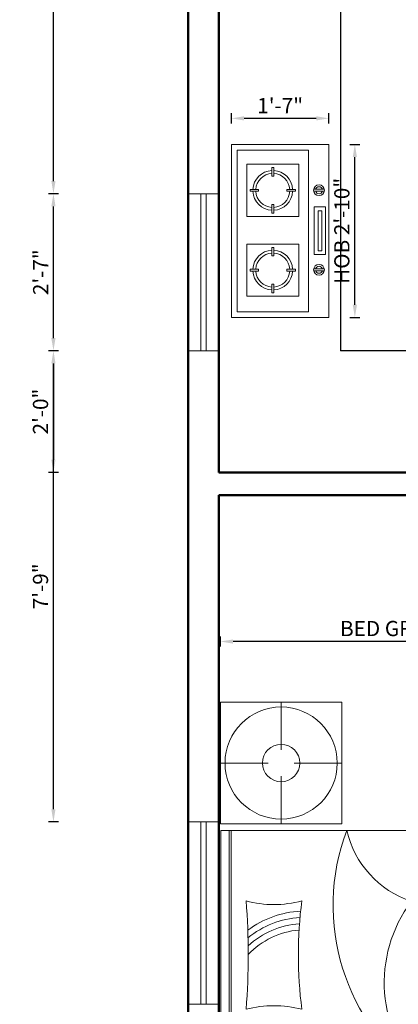
# Model space of a CAD drawing. Units: inches. Extents: x 1961 to 3038, y 800 to 1438.
# Tile 2 of 13: x 2592 to 2666, y 953 to 1148. Entities that reach past the tile are written whole.
import ezdxf

# ---------------------------------------------------------------- set-up
doc = ezdxf.new("R2010")
doc.units = ezdxf.units.IN
for name, color, linetype, lineweight in [('A-ANNO-DIMS', 2, 'Continuous', 18), ('A-EQPM', 8, 'Continuous', 18), ('A-FLOR-CASE', 8, 'Continuous', 25), ('A-FURN', 8, 'Continuous', 18), ('A-GLAZ', 4, 'Continuous', 18), ('A-WALL', 7, 'Continuous', 50)]:
    doc.layers.add(name, color=color, linetype=linetype, lineweight=lineweight)
doc.styles.get("Standard").update_dxf_attribs({"font": 'arial.ttf'})
doc.dimstyles.new('ISO-25', dxfattribs={"dimtxt": 3, "dimasz": 2.5, "dimexe": 1, "dimexo": 1, "dimtad": 1, "dimdec": 4, "dimlunit": 4, "dimtxsty": 'Standard', "dimcen": 2.5, "dimadec": 0, "dimazin": 0, "dimtfac": 1, "dimtdec": 4, "dimtmove": 0, "dimatfit": 3, "dimfxl": 1, "dimfxlon": 1, "dimarcsym": 0})

# ---------------------------------------------------------------- blocks, each defined once
blk = doc.blocks.new('A$C11850ECD')
for p, q in [((0, 1.95), (0, 0.04)), ((0, 1.95), (1.2, 1.95)), ((1.2, 1.95), (1.2, 0.04)), ((1.2318, 1.952), (1.8168, 1.952)), ((1.2318, 1.367), (1.2318, 1.952)), ((1.5243, 1.952), (1.5243, 1.7225)), ((1.8168, 1.952), (1.8168, 1.367)), ((0, 1.91), (1.2, 1.91)), ((0, 1.9), (1.2, 1.9)), ((1.4613, 1.6586), (1.2318, 1.6586)), ((1.8168, 1.6595), (1.5873, 1.6595)), ((1.5243, 1.5965), (1.5243, 1.367)), ((1.8168, 1.367), (1.2318, 1.367)), ((0, 0.58), (1.2, 0.58)), ((0, 0.55), (1.2, 0.55)), ((0, 0.52), (1.2, 0.52)), ((0, 0.49), (1.2, 0.49)), ((0, 0.46), (1.2, 0.46)), ((0, 0.43), (1.2, 0.43)), ((0, 0.4), (1.2, 0.4)), ((1.16, 0), (0.04, 0))]:
    blk.add_line(p, q)
for radius in [0.27, 0.09]:
    blk.add_circle((1.5243, 1.6595), radius)
for centre, radius, start, end in [((-0.2053, 1.694), 0.5605, 346.15, 13.85), ((0.5998, 5.1077), 3.2899, 265.4501, 274.5499), ((0.3425, 1.5416), 0.3789, 4.7708, 46.8165), ((0.3425, 1.5416), 0.4089, 4.1373, 42.5614), ((0.3425, 1.5416), 0.4389, 3.5318, 39.1874), ((0.3425, 1.5416), 0.4689, 2.9489, 36.4321), ((1.3429, 1.694), 0.5004, 164.4468, 195.5532), ((0.5998, -0.4629), 2.0395, 82.6483, 97.3517), ((0.8389, 0.3894), 1.0202, 69.2731, 145.3133), ((1.3044, 0.8859), 0.4695, 102.8515, 161.769), ((0.4655, 0.5058), 0.6574, 53.2823, 135.0802), ((0.04, 0.04), 0.04, 180, 270), ((1.16, 0.04), 0.04, 270, 0)]:
    blk.add_arc(centre, radius, start, end)
blk = doc.blocks.new('A$C056B3B93')
at = {"ltscale": 1000}
for p, q in [((799.8, 450), (0, 450)), ((0, 450), (0, 0)), ((773.3, 423.5), (26.5, 423.5)), ((26.5, 423.5), (26.5, 94.3)), ((773.3, 423.5), (773.3, 94.3)), ((799.8, 450), (799.8, 0)), ((98.6, 379.4), (98.6, 138.4)), ((339.3, 379.4), (98.6, 379.4)), ((223.4, 363.9), (214.5, 363.9)), ((214.5, 324.2), (214.5, 363.9)), ((223.4, 324.2), (223.4, 363.9)), ((339.3, 379.4), (339.3, 138.4)), ((466.7, 379.4), (466.7, 138.4)), ((707.5, 379.4), (466.7, 379.4)), ((591.5, 363.9), (582.7, 363.9)), ((582.7, 324.2), (582.7, 363.9)), ((591.5, 324.2), (591.5, 363.9)), ((707.5, 379.4), (707.5, 138.4)), ((223.4, 324.2), (214.5, 324.2)), ((591.5, 324.2), (582.7, 324.2)), ((114, 263.3), (114, 254.5)), ((153.7, 263.3), (114, 263.3)), ((153.7, 254.5), (114, 254.5)), ((153.7, 254.5), (153.7, 263.3)), ((323.9, 263.3), (284.3, 263.3)), ((284.3, 263.3), (284.3, 254.5)), ((323.9, 254.5), (284.3, 254.5)), ((323.9, 263.3), (323.9, 254.5)), ((482.1, 263.3), (482.1, 254.5)), ((521.8, 263.3), (482.1, 263.3)), ((521.8, 254.5), (482.1, 254.5)), ((521.8, 254.5), (521.8, 263.3)), ((652.4, 263.3), (652.4, 254.5)), ((692.1, 263.3), (652.4, 263.3)), ((692.1, 254.5), (652.4, 254.5)), ((692.1, 263.3), (692.1, 254.5)), ((214.5, 153.9), (214.5, 193.6)), ((223.4, 193.6), (214.5, 193.6)), ((223.4, 153.9), (223.4, 193.6)), ((582.7, 153.9), (582.7, 193.6)), ((591.5, 193.6), (582.7, 193.6)), ((591.5, 153.9), (591.5, 193.6)), ((98.6, 138.4), (339.3, 138.4)), ((223.4, 153.9), (214.5, 153.9)), ((466.7, 138.4), (707.5, 138.4)), ((591.5, 153.9), (582.7, 153.9)), ((26.5, 94.3), (773.3, 94.3)), ((215.7, 69.9), (215.7, 21)), ((224.5, 70), (224.5, 20.9)), ((510.4, 67.7), (290.1, 67.7)), ((290.1, 67.7), (290.1, 15.5)), ((307.7, 50), (307.7, 33.2)), ((492.8, 50), (307.7, 50)), ((492.8, 50), (492.8, 33.2)), ((510.4, 67.7), (510.4, 15.5)), ((583.2, 69.9), (583.2, 21)), ((592, 70), (592, 20.9)), ((799.8, 0), (0, 0)), ((510.4, 15.5), (290.1, 15.5)), ((492.8, 33.2), (307.7, 33.2))]:
    blk.add_line(p, q, dxfattribs=at)
for centre in [(220.2, 45.5), (587.7, 45.5)]:
    blk.add_circle(centre, 24.9, dxfattribs=at)
for centre, radius, start, end in [((219, 258.9), 91.8, 92.7548, 177.2452), ((219, 258.9), 78.5, 93.2193, 176.7807), ((219, 258.9), 91.8, 2.7548, 87.2452), ((219, 258.9), 78.5, 3.2193, 86.7807), ((587.1, 258.9), 91.8, 92.7548, 177.2452), ((587.1, 258.9), 78.5, 93.2193, 176.7807), ((587.1, 258.9), 91.8, 2.7548, 87.2452), ((587.1, 258.9), 78.5, 3.2193, 86.7807), ((219, 258.9), 91.8, 182.7548, 267.2452), ((219, 258.9), 78.5, 183.2193, 266.7807), ((219, 258.9), 78.5, 273.2193, 356.7807), ((219, 258.9), 91.8, 272.7548, 357.2452), ((587.1, 258.9), 91.8, 182.7548, 267.2452), ((587.1, 258.9), 78.5, 183.2193, 266.7807), ((587.1, 258.9), 78.5, 273.2193, 356.7807), ((587.1, 258.9), 91.8, 272.7548, 357.2452), ((220.2, 45.5), 16.1, 106.3425, 253.6575), ((220.2, 45.5), 16.1, 285.5089, 74.4911), ((587.7, 45.5), 16.1, 106.3425, 253.6575), ((587.7, 45.5), 16.1, 285.5089, 74.4911)]:
    blk.add_arc(centre, radius, start, end, dxfattribs=at)
blk = doc.blocks.new('WIN-36IN')
for p, q in [((0, 36), (6, 36)), ((2.5, 36), (2.5, 0)), ((3.5, 36), (3.5, 0)), ((0, 0), (6, 0))]:
    blk.add_line(p, q)
blk = doc.blocks.new('*D57')
at = {"layer": 'A-ANNO-DIMS', "color": 0, "lineweight": -2, "transparency": 16777216}
for p, q in [((2631.09, 1024.03), (2631.09, 1026.03)), ((2708.59, 1025.03), (2633.59, 1025.03)), ((2711.09, 1024.03), (2711.09, 1026.03))]:
    blk.add_line(p, q, dxfattribs=at)
at = {"layer": 'A-ANNO-DIMS', "color": 0, "transparency": 16777216}
for points in [[(2633.59, 1025.44), (2633.59, 1024.61), (2631.09, 1025.03)], [(2708.59, 1025.44), (2708.59, 1024.61), (2711.09, 1025.03)]]:
    blk.add_solid(points, dxfattribs=at)
at = {"layer": 'Defpoints', "color": 0, "transparency": 16777216}
for p in [(2631.09, 1025.03), (2631.09, 1013.03), (2711.09, 1013.03)]:
    blk.add_point(p, dxfattribs=at)
at = {"layer": 'A-ANNO-DIMS', "color": 0, "transparency": 16777216, "insert": (2671.09, 1027.2), "char_height": 3, "attachment_point": 5}
blk.add_mtext('BED GROUP 6\'-8"', dxfattribs=at)
blk = doc.blocks.new('*D67')
at = {"layer": 'A-ANNO-DIMS', "color": 0, "lineweight": -2, "transparency": 16777216}
for p, q in [((2656.61, 1123.16), (2658.61, 1123.16)), ((2657.61, 1091.49), (2657.61, 1120.66)), ((2656.61, 1088.99), (2658.61, 1088.99))]:
    blk.add_line(p, q, dxfattribs=at)
at = {"layer": 'A-ANNO-DIMS', "color": 0, "transparency": 16777216}
for points in [[(2657.2, 1120.66), (2658.03, 1120.66), (2657.61, 1123.16)], [(2657.2, 1091.49), (2658.03, 1091.49), (2657.61, 1088.99)]]:
    blk.add_solid(points, dxfattribs=at)
at = {"layer": 'Defpoints', "color": 0, "transparency": 16777216}
for p in [(2652.49, 1123.16), (2657.61, 1123.16), (2652.49, 1088.99)]:
    blk.add_point(p, dxfattribs=at)
at = {"layer": 'A-ANNO-DIMS', "color": 0, "transparency": 16777216, "insert": (2655.44, 1106.08), "char_height": 3, "attachment_point": 5, "rotation": 90}
blk.add_mtext('HOB 2\'-10"', dxfattribs=at)
blk = doc.blocks.new('*D68')
at = {"layer": 'A-ANNO-DIMS', "color": 0, "lineweight": -2, "transparency": 16777216}
for p, q in [((2633.26, 1127.29), (2633.26, 1129.29)), ((2652.49, 1127.29), (2652.49, 1129.29)), ((2649.99, 1128.29), (2635.76, 1128.29))]:
    blk.add_line(p, q, dxfattribs=at)
at = {"layer": 'A-ANNO-DIMS', "color": 0, "transparency": 16777216}
for points in [[(2635.76, 1128.7), (2635.76, 1127.87), (2633.26, 1128.29)], [(2649.99, 1128.7), (2649.99, 1127.87), (2652.49, 1128.29)]]:
    blk.add_solid(points, dxfattribs=at)
at = {"layer": 'Defpoints', "color": 0, "transparency": 16777216}
for p in [(2633.26, 1128.29), (2633.26, 1123.16), (2652.49, 1123.16)]:
    blk.add_point(p, dxfattribs=at)
at = {"layer": 'A-ANNO-DIMS', "color": 0, "transparency": 16777216, "insert": (2642.88, 1130.42), "char_height": 3, "attachment_point": 5}
blk.add_mtext('1\'-7"', dxfattribs=at)
blk = doc.blocks.new('*D73')
at = {"layer": 'A-ANNO-DIMS', "color": 0, "lineweight": -2, "transparency": 16777216}
for p, q in [((2599.17, 1113.42), (2597.17, 1113.42)), ((2598.17, 1084.92), (2598.17, 1110.92)), ((2599.17, 1082.42), (2597.17, 1082.42))]:
    blk.add_line(p, q, dxfattribs=at)
at = {"layer": 'A-ANNO-DIMS', "color": 0, "transparency": 16777216}
for points in [[(2597.75, 1110.92), (2598.58, 1110.92), (2598.17, 1113.42)], [(2597.75, 1084.92), (2598.58, 1084.92), (2598.17, 1082.42)]]:
    blk.add_solid(points, dxfattribs=at)
at = {"layer": 'Defpoints', "color": 0, "transparency": 16777216}
for p in [(2598.17, 1113.42), (2624.77, 1113.42), (2624.77, 1082.42)]:
    blk.add_point(p, dxfattribs=at)
at = {"layer": 'A-ANNO-DIMS', "color": 0, "transparency": 16777216, "insert": (2596.04, 1097.92), "char_height": 3, "attachment_point": 5, "rotation": 90}
blk.add_mtext('2\'-7"', dxfattribs=at)
blk = doc.blocks.new('*D80')
at = {"layer": 'A-ANNO-DIMS', "color": 0, "lineweight": -2, "transparency": 16777216}
for p, q in [((2599.17, 1200.92), (2597.17, 1200.92)), ((2598.17, 1115.92), (2598.17, 1198.42)), ((2599.17, 1113.42), (2597.17, 1113.42))]:
    blk.add_line(p, q, dxfattribs=at)
at = {"layer": 'A-ANNO-DIMS', "color": 0, "transparency": 16777216}
for points in [[(2597.75, 1198.42), (2598.58, 1198.42), (2598.17, 1200.92)], [(2597.75, 1115.92), (2598.58, 1115.92), (2598.17, 1113.42)]]:
    blk.add_solid(points, dxfattribs=at)
at = {"layer": 'Defpoints', "color": 0, "transparency": 16777216}
for p in [(2598.17, 1200.92), (2624.77, 1200.92), (2624.77, 1113.42)]:
    blk.add_point(p, dxfattribs=at)
at = {"layer": 'A-ANNO-DIMS', "color": 0, "transparency": 16777216, "insert": (2595.99, 1157.17), "char_height": 3, "attachment_point": 5, "rotation": 90}
blk.add_mtext('7\'-3 1/2"', dxfattribs=at)
blk = doc.blocks.new('*D81')
at = {"layer": 'A-ANNO-DIMS', "color": 0, "lineweight": -2, "transparency": 16777216}
for p, q in [((2599.17, 1082.42), (2597.17, 1082.42)), ((2598.17, 991.92), (2598.17, 1079.92)), ((2599.17, 989.42), (2597.17, 989.42))]:
    blk.add_line(p, q, dxfattribs=at)
at = {"layer": 'A-ANNO-DIMS', "color": 0, "transparency": 16777216}
for points in [[(2597.75, 1079.92), (2598.58, 1079.92), (2598.17, 1082.42)], [(2597.75, 991.92), (2598.58, 991.92), (2598.17, 989.42)]]:
    blk.add_solid(points, dxfattribs=at)
at = {"layer": 'Defpoints', "color": 0, "transparency": 16777216}
for p in [(2598.17, 1082.42), (2624.77, 1082.42), (2624.77, 989.42)]:
    blk.add_point(p, dxfattribs=at)
at = {"layer": 'A-ANNO-DIMS', "color": 0, "transparency": 16777216, "insert": (2596.01, 1035.92), "char_height": 3, "attachment_point": 5, "rotation": 90}
blk.add_mtext('7\'-9"', dxfattribs=at)
blk = doc.blocks.new('*D87')
at = {"layer": 'A-ANNO-DIMS', "color": 0, "lineweight": -2, "transparency": 16777216}
for p, q in [((2599.17, 1082.42), (2597.17, 1082.42)), ((2598.17, 1079.92), (2598.17, 1060.92)), ((2599.17, 1058.42), (2597.17, 1058.42))]:
    blk.add_line(p, q, dxfattribs=at)
at = {"layer": 'A-ANNO-DIMS', "color": 0, "transparency": 16777216}
for points in [[(2597.75, 1079.92), (2598.58, 1079.92), (2598.17, 1082.42)], [(2597.75, 1060.92), (2598.58, 1060.92), (2598.17, 1058.42)]]:
    blk.add_solid(points, dxfattribs=at)
at = {"layer": 'Defpoints', "color": 0, "transparency": 16777216}
for p in [(2654.77, 1082.42), (2598.17, 1058.42), (2630.77, 1058.42)]:
    blk.add_point(p, dxfattribs=at)
at = {"layer": 'A-ANNO-DIMS', "color": 0, "transparency": 16777216, "insert": (2596.01, 1070.42), "char_height": 3, "attachment_point": 5, "rotation": 90}
blk.add_mtext('2\'-0"', dxfattribs=at)

msp = doc.modelspace()

# ---------------------------------------------------------------- linework, layer by layer
at = {"layer": 'A-FLOR-CASE'}
for p in [(2654.76803, 1160.41975), (2726.76803, 1082.41975)]:
    msp.add_line(p, (2654.76803, 1082.41975), dxfattribs=at)
at = {"layer": 'A-GLAZ'}
for p, q in [((2630.76803, 1113.41975), (2624.76803, 1113.41975)), ((2627.26803, 1113.41975), (2627.26803, 1082.41975)), ((2628.26803, 1113.41975), (2628.26803, 1082.41975)), ((2630.76803, 1082.41975), (2624.76803, 1082.41975))]:
    msp.add_line(p, q, dxfattribs=at)
at = {"layer": 'A-WALL'}
for p, q in [((2624.76803, 1314.91975), (2624.76803, 852.91975)), ((2630.76803, 1160.41975), (2630.76803, 1058.41975)), ((2726.76803, 1058.41975), (2630.76803, 1058.41975)), ((2759.76803, 1053.91975), (2630.76803, 1053.91975)), ((2630.76803, 1053.91975), (2630.76803, 905.41975))]:
    msp.add_line(p, q, dxfattribs=at)

# ---------------------------------------------------------------- block references
at = {"layer": 'A-EQPM', "xscale": 0.0427221287027107, "yscale": 0.0427221287027107, "zscale": 0.0427221287027107, "rotation": 90}
msp.add_blockref('A$C056B3B93', (2652.48939, 1088.99087), dxfattribs=at)
at = {"layer": 'A-FURN', "xscale": 40.98381615062051, "yscale": 40.98381615062051, "zscale": 40.98381615062051, "rotation": 90}
msp.add_blockref('A$C11850ECD', (2711.08548, 938.57032), dxfattribs=at)
at = {"layer": 'A-GLAZ'}
msp.add_blockref('WIN-36IN', (2624.768, 953.42), dxfattribs=at)

# ---------------------------------------------------------------- dimensions: what is measured, and where the dimension line sits
at = {"layer": 'A-ANNO-DIMS'}
for base, p1, p2, angle, picture, middle in [((2598.16803, 1200.91975), (2624.76803, 1113.41975), (2624.76803, 1200.91975), 90, '*D80', (2595.99085, 1157.16975)), ((2633.26443, 1128.28541), (2652.48938, 1123.16003), (2633.26443, 1123.16003), 180, '*D68', (2642.87691, 1130.41654)), ((2598.16803, 1113.41975), (2624.76803, 1082.41975), (2624.76803, 1113.41975), 90, '*D73', (2596.03689, 1097.91975)), ((2598.16803, 1082.41975), (2624.76803, 989.41975), (2624.76803, 1082.41975), 90, '*D81', (2596.01131, 1035.91975)), ((2598.16803, 1058.41975), (2654.76803, 1082.41975), (2630.76803, 1058.41975), 90, '*D87', (2596.01131, 1070.41975))]:
    dim = msp.add_linear_dim(base=base, p1=p1, p2=p2, angle=angle, dimstyle='ISO-25', override={"dimdec": 1, "dimlfac": 1, "dimrnd": 0, "dimzin": 1, "dimdsep": 46, "dimlunit": 4, "dimfrac": 2}, dxfattribs=at)
    dim.commit()
    dim.dimension.update_dxf_attribs({"geometry": picture, "text_midpoint": middle})
for base, p1, p2, angle, text, picture, middle in [((2657.61476, 1123.16003), (2652.48938, 1088.99087), (2652.48938, 1123.16003), 90, 'HOB <>', '*D67', (2655.43758, 1106.07545)), ((2631.08548, 1025.02777), (2711.08548, 1013.02777), (2631.08548, 1013.02777), 180, 'BED GROUP <>', '*D57', (2671.08548, 1027.20495))]:
    dim = msp.add_linear_dim(base=base, p1=p1, p2=p2, angle=angle, text=text, dimstyle='ISO-25', override={"dimdec": 1, "dimlfac": 1, "dimrnd": 0, "dimzin": 1, "dimdsep": 46, "dimlunit": 4, "dimfrac": 2}, dxfattribs=at)
    dim.commit()
    dim.dimension.update_dxf_attribs({"geometry": picture, "text_midpoint": middle})

doc.saveas('drawing.dxf')
